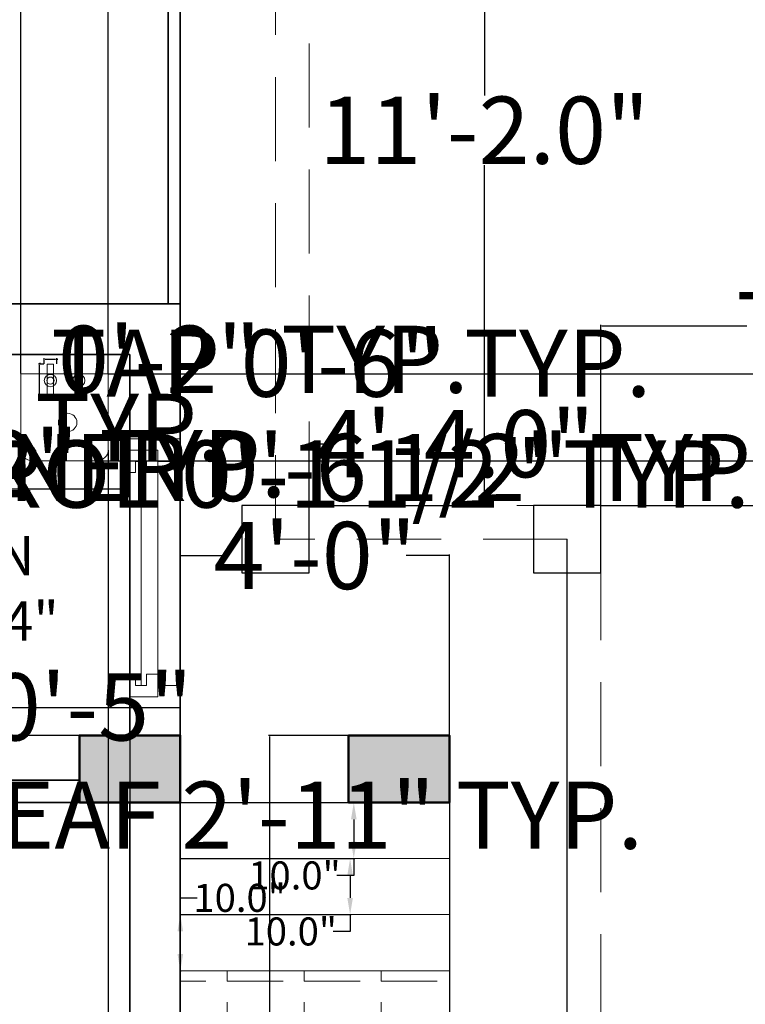
# Model space of a CAD drawing. Units: inches. Extents: x 1063 to 2718, y 423 to 1923.
# Tile 5 of 7: x 1379 to 1509, y 862 to 1038. Entities that reach past the tile are written whole.
import ezdxf

# ---------------------------------------------------------------- set-up
doc = ezdxf.new("R2010")
doc.units = ezdxf.units.IN
doc.header["$LTSCALE"] = 6
doc.header["$MEASUREMENT"] = 0
doc.linetypes.add('HIDDEN', pattern=[0.375, 0.25, -0.125])
for name, color, linetype, lineweight in [('A-ANNO-DIMS', 2, 'Continuous', 18), ('A-AREA-IDEN', 7, 'Continuous', 18), ('A-COLS', 7, 'Continuous', 50), ('A-COLS-PATT', 252, 'Continuous', 13), ('A-FLOR', 7, 'Continuous', 25), ('A-FLOR-CASE', 7, 'Continuous', 25), ('A-FLOR-FIXT', 4, 'Continuous', 18), ('A-FLOR-PATT', 9, 'Continuous', 13), ('A-FLOR-STRS', 7, 'Continuous', 18), ('A-GLAZ', 4, 'Continuous', 18), ('A-WALL', 7, 'Continuous', 35), ('C-PROP', 7, 'Continuous', 25), ('C-PROP-HIDN', 7, 'HIDDEN', 18)]:
    doc.layers.add(name, color=color, linetype=linetype, lineweight=lineweight)
doc.styles.get("Standard").update_dxf_attribs({"font": 'arial.ttf'})
doc.dimstyles.get("Standard").update_dxf_attribs({"dimtxt": 12, "dimasz": 0.18, "dimexe": 0.18, "dimexo": 0.0625, "dimgap": 0.09, "dimtad": 0, "dimtih": 1, "dimtoh": 1, "dimdec": 1, "dimzin": 0, "dimdsep": 46, "dimlunit": 3, "dimtxsty": 'Standard', "dimcen": 0.09, "dimadec": 0, "dimazin": 0, "dimtfac": 1, "dimtdec": 1, "dimtofl": 0, "dimtmove": 0, "dimatfit": 3, "dimfxl": 1, "dimtolj": 1, "dimtzin": 0, "dimarcsym": 0})

# ---------------------------------------------------------------- blocks, each defined once
blk = doc.blocks.new('*D3')
at = {"layer": 'A-ANNO-DIMS', "color": 0, "lineweight": -2, "ltscale": 6, "transparency": 16777216}
for p, q in [((1482.99, 951.12), (1516.18, 951.12)), ((1516, 950.94), (1516, 765.34)), ((1516, 567.3), (1516, 752.9)), ((1482.99, 567.12), (1516.18, 567.12))]:
    blk.add_line(p, q, dxfattribs=at)
at = {"layer": 'A-ANNO-DIMS', "color": 0, "ltscale": 6, "transparency": 16777216}
for points in [[(1515.97, 950.94), (1516.03, 950.94), (1516, 951.12)], [(1515.97, 567.3), (1516.03, 567.3), (1516, 567.12)]]:
    blk.add_solid(points, dxfattribs=at)
at = {"layer": 'Defpoints', "color": 0, "ltscale": 6, "transparency": 16777216}
for p in [(1482.93, 951.12), (1516, 951.12), (1482.93, 567.12)]:
    blk.add_point(p, dxfattribs=at)
at = {"layer": 'A-ANNO-DIMS', "color": 0, "ltscale": 6, "transparency": 16777216, "insert": (1516, 759.12), "char_height": 12, "attachment_point": 5}
blk.add_mtext("\\A1;32'", dxfattribs=at)
blk = doc.blocks.new('*D4')
at = {"layer": 'A-ANNO-DIMS', "color": 0, "lineweight": -2, "ltscale": 6, "transparency": 16777216}
for p, q in [((1430.93, 951.18), (1430.93, 962.35)), ((1431.11, 962.17), (1433.65, 962.17)), ((1482.75, 962.17), (1480.2, 962.17)), ((1482.93, 951.18), (1482.93, 962.35))]:
    blk.add_line(p, q, dxfattribs=at)
at = {"layer": 'A-ANNO-DIMS', "color": 0, "ltscale": 6, "transparency": 16777216}
for points in [[(1431.11, 962.2), (1431.11, 962.14), (1430.93, 962.17)], [(1482.75, 962.2), (1482.75, 962.14), (1482.93, 962.17)]]:
    blk.add_solid(points, dxfattribs=at)
at = {"layer": 'Defpoints', "color": 0, "ltscale": 6, "transparency": 16777216}
for p in [(1430.93, 962.17), (1430.93, 951.12), (1482.93, 951.12)]:
    blk.add_point(p, dxfattribs=at)
at = {"layer": 'A-ANNO-DIMS', "color": 0, "ltscale": 6, "transparency": 16777216, "insert": (1456.93, 962.17), "char_height": 12, "attachment_point": 5}
blk.add_mtext('\\A1;4\'-4.0"', dxfattribs=at)
blk = doc.blocks.new('*D5')
at = {"layer": 'A-ANNO-DIMS', "color": 0, "lineweight": -2, "ltscale": 6, "transparency": 16777216}
for p, q in [((1430.99, 1085.12), (1462.35, 1085.12)), ((1462.17, 1084.94), (1462.17, 1024.34)), ((1462.17, 951.3), (1462.17, 1011.9)), ((1430.99, 951.12), (1462.35, 951.12))]:
    blk.add_line(p, q, dxfattribs=at)
at = {"layer": 'A-ANNO-DIMS', "color": 0, "ltscale": 6, "transparency": 16777216}
for points in [[(1462.14, 1084.94), (1462.2, 1084.94), (1462.17, 1085.12)], [(1462.14, 951.3), (1462.2, 951.3), (1462.17, 951.12)]]:
    blk.add_solid(points, dxfattribs=at)
at = {"layer": 'Defpoints', "color": 0, "ltscale": 6, "transparency": 16777216}
for p in [(1430.93, 1085.12), (1462.17, 1085.12), (1430.93, 951.12)]:
    blk.add_point(p, dxfattribs=at)
at = {"layer": 'A-ANNO-DIMS', "color": 0, "ltscale": 6, "transparency": 16777216, "insert": (1462.17, 1018.12), "char_height": 12, "attachment_point": 5}
blk.add_mtext('\\A1;11\'-2.0"', dxfattribs=at)
blk = doc.blocks.new('*D8')
at = {"layer": 'A-ANNO-DIMS', "color": 0, "lineweight": -2, "ltscale": 6, "transparency": 16777216}
for p, q in [((1407.99, 898.12), (1439.05, 898.12)), ((1438.87, 895.12), (1438.87, 891.12)), ((1407.99, 888.12), (1439.05, 888.12)), ((1438.87, 888.12), (1438.87, 885.12)), ((1438.87, 885.12), (1435.87, 885.12))]:
    blk.add_line(p, q, dxfattribs=at)
at = {"layer": 'A-ANNO-DIMS', "color": 0, "ltscale": 6, "transparency": 16777216}
for points in [[(1438.37, 895.12), (1439.37, 895.12), (1438.87, 898.12)], [(1438.37, 891.12), (1439.37, 891.12), (1438.87, 888.12)]]:
    blk.add_solid(points, dxfattribs=at)
at = {"layer": 'Defpoints', "color": 0, "ltscale": 6, "transparency": 16777216}
for p in [(1407.93, 898.12), (1407.93, 888.12), (1438.87, 888.12)]:
    blk.add_point(p, dxfattribs=at)
at = {"layer": 'A-ANNO-DIMS', "color": 0, "ltscale": 6, "transparency": 16777216, "insert": (1428.29, 885.12), "char_height": 5, "attachment_point": 5}
blk.add_mtext('\\A1;10.0"', dxfattribs=at)
blk = doc.blocks.new('*D9')
at = {"layer": 'A-ANNO-DIMS', "color": 0, "lineweight": -2, "ltscale": 6, "transparency": 16777216}
for p, q in [((1407.99, 888.12), (1438.39, 888.12)), ((1438.21, 885.12), (1438.21, 881.12)), ((1407.99, 878.12), (1438.39, 878.12)), ((1438.21, 878.12), (1438.21, 875.12)), ((1438.21, 875.12), (1435.21, 875.12))]:
    blk.add_line(p, q, dxfattribs=at)
at = {"layer": 'A-ANNO-DIMS', "color": 0, "ltscale": 6, "transparency": 16777216}
for points in [[(1437.71, 885.12), (1438.71, 885.12), (1438.21, 888.12)], [(1437.71, 881.12), (1438.71, 881.12), (1438.21, 878.12)]]:
    blk.add_solid(points, dxfattribs=at)
at = {"layer": 'Defpoints', "color": 0, "ltscale": 6, "transparency": 16777216}
for p in [(1407.93, 888.12), (1407.93, 878.12), (1438.21, 878.12)]:
    blk.add_point(p, dxfattribs=at)
at = {"layer": 'A-ANNO-DIMS', "color": 0, "ltscale": 6, "transparency": 16777216, "insert": (1427.63, 875.12), "char_height": 5, "attachment_point": 5}
blk.add_mtext('\\A1;10.0"', dxfattribs=at)
blk = doc.blocks.new('*D10')
at = {"layer": 'A-ANNO-DIMS', "color": 0, "lineweight": -2, "ltscale": 6, "transparency": 16777216}
for p, q in [((1407.93, 878.12), (1407.93, 881.12)), ((1407.93, 881.12), (1410.93, 881.12)), ((1407.99, 878.12), (1408.11, 878.12)), ((1407.93, 871.12), (1407.93, 875.12)), ((1407.99, 868.12), (1408.11, 868.12))]:
    blk.add_line(p, q, dxfattribs=at)
at = {"layer": 'A-ANNO-DIMS', "color": 0, "ltscale": 6, "transparency": 16777216}
for points in [[(1407.43, 875.12), (1408.43, 875.12), (1407.93, 878.12)], [(1407.43, 871.12), (1408.43, 871.12), (1407.93, 868.12)]]:
    blk.add_solid(points, dxfattribs=at)
at = {"layer": 'Defpoints', "color": 0, "ltscale": 6, "transparency": 16777216}
for p in [(1407.93, 878.12), (1407.93, 878.12), (1407.93, 868.12)]:
    blk.add_point(p, dxfattribs=at)
at = {"layer": 'A-ANNO-DIMS', "color": 0, "ltscale": 6, "transparency": 16777216, "insert": (1418.51, 881.12), "char_height": 5, "attachment_point": 5}
blk.add_mtext('\\A1;10.0"', dxfattribs=at)
blk = doc.blocks.new('WIN-48-SLIDING')
at = {"ltscale": 6}
for p, q in [((0, 9), (4, 9)), ((4, 9), (4, 5)), ((48, 9), (44, 9)), ((44, 9), (44, 5)), ((4, 5), (2, 5)), ((2, 5), (2, 0)), ((4, 5), (44, 5)), ((4, 5), (6, 5)), ((6, 5), (6, 3)), ((44, 5), (42, 5)), ((42, 5), (42, 3)), ((44, 5), (46, 5)), ((46, 5), (46, 0)), ((6, 3), (4, 3)), ((4, 3), (4, 1)), ((4, 2), (44, 2)), ((42, 3), (44, 3)), ((44, 3), (44, 1)), ((4, 1), (6, 1)), ((6, 1), (6, 0)), ((44, 1), (42, 1)), ((42, 1), (42, 0)), ((48, 0), (0, 0)), ((2, 0), (46, 0))]:
    blk.add_line(p, q, dxfattribs=at)
blk.add_lwpolyline([(48, 0), (48, 9), (0, 9), (0, 0)], dxfattribs=at)
blk = doc.blocks.new('COLUMN-18X12')
blk.add_lwpolyline([(0, 0), (18, 0), (18, 12), (0, 12)], close=True)
blk = doc.blocks.new('PIER-12X12')
blk.add_lwpolyline([(0, 0), (12, 0), (12, 12), (0, 12)], close=True)
blk = doc.blocks.new('SINK-TAP')
at = {"ltscale": 6}
blk.add_lwpolyline([(0.54, 5.85), (1.67, 5.85), (1.67, 0), (0.54, 0)], close=True, dxfattribs=at)
for radius in [1.1, 1.1, 0.637]:
    blk.add_circle((1.1, 2.92), radius, dxfattribs=at)
blk = doc.blocks.new('*D34')
at = {"layer": 'A-ANNO-DIMS', "color": 0, "lineweight": -2, "ltscale": 6, "transparency": 16777216}
for p, q in [((1323.62, 956.91), (1323.62, 956.58)), ((1323.8, 956.76), (1324.88, 956.76)), ((1325.06, 956.91), (1325.06, 956.58)), ((1325.06, 956.76), (1325.24, 956.76))]:
    blk.add_line(p, q, dxfattribs=at)
at = {"layer": 'A-ANNO-DIMS', "color": 0, "ltscale": 6, "transparency": 16777216}
for points in [[(1323.8, 956.79), (1323.8, 956.73), (1323.62, 956.76)], [(1324.88, 956.79), (1324.88, 956.73), (1325.06, 956.76)]]:
    blk.add_solid(points, dxfattribs=at)
at = {"layer": 'Defpoints', "color": 0, "ltscale": 6, "transparency": 16777216}
for p in [(1323.62, 956.97), (1325.06, 956.97), (1325.06, 956.76)]:
    blk.add_point(p, dxfattribs=at)
at = {"layer": 'A-ANNO-DIMS', "color": 0, "ltscale": 6, "transparency": 16777216, "insert": (1419.12, 956.76), "char_height": 12, "attachment_point": 5}
blk.add_mtext('\\A1;CONTROL 0\'-1 1/2" TYP.', dxfattribs=at)
blk = doc.blocks.new('*D35')
at = {"layer": 'A-ANNO-DIMS', "color": 0, "lineweight": -2, "ltscale": 6, "transparency": 16777216}
for p, q in [((1325.12, 958.41), (1325.45, 958.41)), ((1325.27, 958.41), (1325.27, 958.59)), ((1325.27, 958.59), (1325.45, 958.59)), ((1325.27, 957.15), (1325.27, 958.23)), ((1325.12, 956.97), (1325.45, 956.97))]:
    blk.add_line(p, q, dxfattribs=at)
at = {"layer": 'A-ANNO-DIMS', "color": 0, "ltscale": 6, "transparency": 16777216}
for points in [[(1325.24, 958.23), (1325.3, 958.23), (1325.27, 958.41)], [(1325.24, 957.15), (1325.3, 957.15), (1325.27, 956.97)]]:
    blk.add_solid(points, dxfattribs=at)
at = {"layer": 'Defpoints', "color": 0, "ltscale": 6, "transparency": 16777216}
for p in [(1325.06, 958.41), (1325.27, 958.41), (1325.06, 956.97)]:
    blk.add_point(p, dxfattribs=at)
at = {"layer": 'A-ANNO-DIMS', "color": 0, "ltscale": 6, "transparency": 16777216, "insert": (1376.1, 958.59), "char_height": 12, "attachment_point": 5}
blk.add_mtext('\\A1;0\'-1 1/2" TYP.', dxfattribs=at)
blk = doc.blocks.new('*D36')
at = {"layer": 'A-ANNO-DIMS', "color": 0, "lineweight": -2, "ltscale": 6, "transparency": 16777216}
for p, q in [((1334.27, 958.87), (1334.27, 957.74)), ((1334.45, 957.92), (1340.83, 957.92)), ((1341.01, 958.87), (1341.01, 957.74)), ((1341.01, 957.92), (1341.19, 957.92))]:
    blk.add_line(p, q, dxfattribs=at)
at = {"layer": 'A-ANNO-DIMS', "color": 0, "ltscale": 6, "transparency": 16777216}
for points in [[(1334.45, 957.95), (1334.45, 957.89), (1334.27, 957.92)], [(1340.83, 957.95), (1340.83, 957.89), (1341.01, 957.92)]]:
    blk.add_solid(points, dxfattribs=at)
at = {"layer": 'Defpoints', "color": 0, "ltscale": 6, "transparency": 16777216}
for p in [(1334.27, 958.93), (1341.01, 958.93), (1341.01, 957.92)]:
    blk.add_point(p, dxfattribs=at)
at = {"layer": 'A-ANNO-DIMS', "color": 0, "ltscale": 6, "transparency": 16777216, "insert": (1429.29, 957.92), "char_height": 12, "attachment_point": 5}
blk.add_mtext('\\A1;BURNER 0\'-6 1/2" TYP.', dxfattribs=at)
blk = doc.blocks.new('*D37')
at = {"layer": 'A-ANNO-DIMS', "color": 0, "lineweight": -2, "ltscale": 6, "transparency": 16777216}
for p, q in [((1341.07, 964.9), (1342.2, 964.9)), ((1342.02, 964.9), (1342.02, 965.08)), ((1342.02, 965.08), (1342.2, 965.08)), ((1342.02, 959.11), (1342.02, 964.72)), ((1341.07, 958.93), (1342.2, 958.93))]:
    blk.add_line(p, q, dxfattribs=at)
at = {"layer": 'A-ANNO-DIMS', "color": 0, "ltscale": 6, "transparency": 16777216}
for points in [[(1341.99, 964.72), (1342.05, 964.72), (1342.02, 964.9)], [(1341.99, 959.11), (1342.05, 959.11), (1342.02, 958.93)]]:
    blk.add_solid(points, dxfattribs=at)
at = {"layer": 'Defpoints', "color": 0, "ltscale": 6, "transparency": 16777216}
for p in [(1341.01, 964.9), (1342.02, 964.9), (1341.01, 958.93)]:
    blk.add_point(p, dxfattribs=at)
at = {"layer": 'A-ANNO-DIMS', "color": 0, "ltscale": 6, "transparency": 16777216, "insert": (1378.86, 965.08), "char_height": 12, "attachment_point": 5}
blk.add_mtext('\\A1;0\'-6" TYP.', dxfattribs=at)
blk = doc.blocks.new('*D38')
at = {"layer": 'A-ANNO-DIMS', "color": 0, "lineweight": -2, "ltscale": 6, "transparency": 16777216}
for p, q in [((1383.61, 976.37), (1382.62, 976.37)), ((1382.8, 976.37), (1382.8, 976.55)), ((1382.8, 976.55), (1382.98, 976.55)), ((1382.8, 970.7), (1382.8, 976.19)), ((1383.61, 970.52), (1382.62, 970.52))]:
    blk.add_line(p, q, dxfattribs=at)
at = {"layer": 'A-ANNO-DIMS', "color": 0, "ltscale": 6, "transparency": 16777216}
for points in [[(1382.77, 976.19), (1382.83, 976.19), (1382.8, 976.37)], [(1382.77, 970.7), (1382.83, 970.7), (1382.8, 970.52)]]:
    blk.add_solid(points, dxfattribs=at)
at = {"layer": 'Defpoints', "color": 0, "ltscale": 6, "transparency": 16777216}
for p in [(1382.8, 976.37), (1383.67, 976.37), (1383.67, 970.52)]:
    blk.add_point(p, dxfattribs=at)
at = {"layer": 'A-ANNO-DIMS', "color": 0, "ltscale": 6, "transparency": 16777216, "insert": (1438.42, 976.55), "char_height": 12, "attachment_point": 5}
blk.add_mtext('\\A1;TAP 0\'-6" TYP.', dxfattribs=at)
blk = doc.blocks.new('*D39')
at = {"layer": 'A-ANNO-DIMS', "color": 0, "lineweight": -2, "ltscale": 6, "transparency": 16777216}
for p, q in [((1383.67, 976.43), (1383.67, 977.42)), ((1383.85, 977.24), (1385.7, 977.24)), ((1385.88, 976.43), (1385.88, 977.42)), ((1385.88, 977.24), (1386.06, 977.24))]:
    blk.add_line(p, q, dxfattribs=at)
at = {"layer": 'A-ANNO-DIMS', "color": 0, "ltscale": 6, "transparency": 16777216}
for points in [[(1383.85, 977.27), (1383.85, 977.21), (1383.67, 977.24)], [(1385.7, 977.27), (1385.7, 977.21), (1385.88, 977.24)]]:
    blk.add_solid(points, dxfattribs=at)
at = {"layer": 'Defpoints', "color": 0, "ltscale": 6, "transparency": 16777216}
for p in [(1385.88, 977.24), (1383.67, 976.37), (1385.88, 976.37)]:
    blk.add_point(p, dxfattribs=at)
at = {"layer": 'A-ANNO-DIMS', "color": 0, "ltscale": 6, "transparency": 16777216, "insert": (1422.73, 977.24), "char_height": 12, "attachment_point": 5}
blk.add_mtext('\\A1;0\'-2" TYP.', dxfattribs=at)
blk = doc.blocks.new('*D42')
at = {"layer": 'A-ANNO-DIMS', "color": 0, "lineweight": -2, "ltscale": 6, "transparency": 16777216}
for p, q in [((1265.93, 901.06), (1265.93, 895.69)), ((1300.93, 901.06), (1300.93, 895.69)), ((1266.11, 895.87), (1300.75, 895.87)), ((1300.93, 895.87), (1301.11, 895.87))]:
    blk.add_line(p, q, dxfattribs=at)
at = {"layer": 'A-ANNO-DIMS', "color": 0, "ltscale": 6, "transparency": 16777216}
for points in [[(1266.11, 895.9), (1266.11, 895.84), (1265.93, 895.87)], [(1300.75, 895.9), (1300.75, 895.84), (1300.93, 895.87)]]:
    blk.add_solid(points, dxfattribs=at)
at = {"layer": 'Defpoints', "color": 0, "ltscale": 6, "transparency": 16777216}
for p in [(1265.93, 901.12), (1300.93, 901.12), (1300.93, 895.87)]:
    blk.add_point(p, dxfattribs=at)
at = {"layer": 'A-ANNO-DIMS', "color": 0, "ltscale": 6, "transparency": 16777216, "insert": (1398.77, 895.87), "char_height": 12, "attachment_point": 5}
blk.add_mtext('\\A1;SINGLE LEAF 2\'-11" TYP.', dxfattribs=at)
blk = doc.blocks.new('*D48')
at = {"layer": 'A-ANNO-DIMS', "color": 0, "lineweight": -2, "ltscale": 6, "transparency": 16777216}
for p, q in [((1482.93, 951.18), (1482.93, 983.4)), ((1483.11, 983.22), (1508.94, 983.22)), ((1566.75, 983.22), (1540.92, 983.22)), ((1566.93, 951.18), (1566.93, 983.4))]:
    blk.add_line(p, q, dxfattribs=at)
at = {"layer": 'A-ANNO-DIMS', "color": 0, "ltscale": 6, "transparency": 16777216}
for points in [[(1483.11, 983.25), (1483.11, 983.19), (1482.93, 983.22)], [(1566.75, 983.25), (1566.75, 983.19), (1566.93, 983.22)]]:
    blk.add_solid(points, dxfattribs=at)
at = {"layer": 'Defpoints', "color": 0, "ltscale": 6, "transparency": 16777216}
for p in [(1566.93, 983.22), (1482.93, 951.12), (1566.93, 951.12)]:
    blk.add_point(p, dxfattribs=at)
at = {"layer": 'A-ANNO-DIMS', "color": 0, "ltscale": 6, "transparency": 16777216, "insert": (1524.93, 983.22), "char_height": 12, "attachment_point": 5}
blk.add_mtext('\\A1;7\'-0"', dxfattribs=at)
blk = doc.blocks.new('*D51')
at = {"layer": 'A-ANNO-DIMS', "color": 0, "lineweight": -2, "ltscale": 6, "transparency": 16777216}
for p, q in [((1407.93, 910.18), (1407.93, 942.4)), ((1408.11, 942.22), (1415.64, 942.22)), ((1455.75, 942.22), (1448.21, 942.22)), ((1455.93, 910.18), (1455.93, 942.4))]:
    blk.add_line(p, q, dxfattribs=at)
at = {"layer": 'A-ANNO-DIMS', "color": 0, "ltscale": 6, "transparency": 16777216}
for points in [[(1408.11, 942.25), (1408.11, 942.19), (1407.93, 942.22)], [(1455.75, 942.25), (1455.75, 942.19), (1455.93, 942.22)]]:
    blk.add_solid(points, dxfattribs=at)
at = {"layer": 'Defpoints', "color": 0, "ltscale": 6, "transparency": 16777216}
for p in [(1455.93, 942.22), (1407.93, 910.12), (1455.93, 910.12)]:
    blk.add_point(p, dxfattribs=at)
at = {"layer": 'A-ANNO-DIMS', "color": 0, "ltscale": 6, "transparency": 16777216, "insert": (1431.93, 942.22), "char_height": 12, "attachment_point": 5}
blk.add_mtext('\\A1;4\'-0"', dxfattribs=at)
blk = doc.blocks.new('*D52')
at = {"layer": 'A-ANNO-DIMS', "color": 0, "lineweight": -2, "ltscale": 6, "transparency": 16777216}
for p, q in [((1455.86, 910.12), (1423.65, 910.12)), ((1423.83, 909.94), (1423.83, 756.84)), ((1423.83, 591.3), (1423.83, 744.4)), ((1455.86, 591.12), (1423.65, 591.12))]:
    blk.add_line(p, q, dxfattribs=at)
at = {"layer": 'A-ANNO-DIMS', "color": 0, "ltscale": 6, "transparency": 16777216}
for points in [[(1423.8, 909.94), (1423.86, 909.94), (1423.83, 910.12)], [(1423.8, 591.3), (1423.86, 591.3), (1423.83, 591.12)]]:
    blk.add_solid(points, dxfattribs=at)
at = {"layer": 'Defpoints', "color": 0, "ltscale": 6, "transparency": 16777216}
for p in [(1423.83, 910.12), (1455.93, 910.12), (1455.93, 591.12)]:
    blk.add_point(p, dxfattribs=at)
at = {"layer": 'A-ANNO-DIMS', "color": 0, "ltscale": 6, "transparency": 16777216, "insert": (1423.83, 750.62), "char_height": 12, "attachment_point": 5}
blk.add_mtext('\\A1;26\'-7"', dxfattribs=at)
blk = doc.blocks.new('*D60')
at = {"layer": 'A-ANNO-DIMS', "color": 0, "lineweight": -2, "ltscale": 6, "transparency": 16777216}
for p, q in [((1321.21, 974.62), (1321.21, 1117.4)), ((1321.39, 1117.22), (1342.7, 1117.22)), ((1342.88, 974.62), (1342.88, 1117.4)), ((1342.88, 1117.22), (1343.06, 1117.22))]:
    blk.add_line(p, q, dxfattribs=at)
at = {"layer": 'A-ANNO-DIMS', "color": 0, "ltscale": 6, "transparency": 16777216}
for points in [[(1321.39, 1117.25), (1321.39, 1117.19), (1321.21, 1117.22)], [(1342.7, 1117.25), (1342.7, 1117.19), (1342.88, 1117.22)]]:
    blk.add_solid(points, dxfattribs=at)
at = {"layer": 'Defpoints', "color": 0, "ltscale": 6, "transparency": 16777216}
for p in [(1342.88, 1117.22), (1321.21, 974.55), (1342.88, 974.55)]:
    blk.add_point(p, dxfattribs=at)
at = {"layer": 'A-ANNO-DIMS', "color": 0, "ltscale": 6, "transparency": 16777216, "insert": (1372.52, 1117.22), "char_height": 12, "attachment_point": 5}
blk.add_mtext('\\A1;1\'-9 1/2"', dxfattribs=at)
blk = doc.blocks.new('*D62')
at = {"layer": 'A-ANNO-DIMS', "color": 0, "lineweight": -2, "ltscale": 6, "transparency": 16777216}
for p, q in [((1379.5, 974.73), (1379.5, 1117.4)), ((1379.68, 1117.22), (1394.9, 1117.22)), ((1395.08, 974.73), (1395.08, 1117.4)), ((1395.08, 1117.22), (1395.26, 1117.22))]:
    blk.add_line(p, q, dxfattribs=at)
at = {"layer": 'A-ANNO-DIMS', "color": 0, "ltscale": 6, "transparency": 16777216}
for points in [[(1379.68, 1117.25), (1379.68, 1117.19), (1379.5, 1117.22)], [(1394.9, 1117.25), (1394.9, 1117.19), (1395.08, 1117.22)]]:
    blk.add_solid(points, dxfattribs=at)
at = {"layer": 'Defpoints', "color": 0, "ltscale": 6, "transparency": 16777216}
for p in [(1395.08, 1117.22), (1379.5, 974.67), (1395.08, 974.67)]:
    blk.add_point(p, dxfattribs=at)
at = {"layer": 'A-ANNO-DIMS', "color": 0, "ltscale": 6, "transparency": 16777216, "insert": (1424.71, 1117.22), "char_height": 12, "attachment_point": 5}
blk.add_mtext('\\A1;1\'-3 1/2"', dxfattribs=at)
blk = doc.blocks.new('*D63')
at = {"layer": 'A-ANNO-DIMS', "color": 0, "lineweight": -2, "ltscale": 6, "transparency": 16777216}
for p, q in [((1395.14, 974.67), (1599.21, 974.67)), ((1599.03, 974.49), (1599.03, 973.19)), ((1599.03, 959.29), (1599.03, 960.59)), ((1393.14, 959.11), (1599.21, 959.11))]:
    blk.add_line(p, q, dxfattribs=at)
at = {"layer": 'A-ANNO-DIMS', "color": 0, "ltscale": 6, "transparency": 16777216}
for points in [[(1599, 974.49), (1599.06, 974.49), (1599.03, 974.67)], [(1599, 959.29), (1599.06, 959.29), (1599.03, 959.11)]]:
    blk.add_solid(points, dxfattribs=at)
at = {"layer": 'Defpoints', "color": 0, "ltscale": 6, "transparency": 16777216}
for p in [(1395.08, 974.67), (1393.08, 959.11), (1599.03, 959.11)]:
    blk.add_point(p, dxfattribs=at)
at = {"layer": 'A-ANNO-DIMS', "color": 0, "ltscale": 6, "transparency": 16777216, "insert": (1599.03, 966.89), "char_height": 12, "attachment_point": 5}
blk.add_mtext('\\A1;1\'-3 1/2"', dxfattribs=at)
blk = doc.blocks.new('*D64')
at = {"layer": 'A-ANNO-DIMS', "color": 0, "lineweight": -2, "ltscale": 6, "transparency": 16777216}
for p, q in [((1310.93, 978.18), (1310.93, 1117.4)), ((1311.11, 1117.22), (1321.03, 1117.22)), ((1321.21, 974.62), (1321.21, 1117.4)), ((1321.21, 1117.22), (1321.39, 1117.22))]:
    blk.add_line(p, q, dxfattribs=at)
at = {"layer": 'A-ANNO-DIMS', "color": 0, "ltscale": 6, "transparency": 16777216}
for points in [[(1311.11, 1117.25), (1311.11, 1117.19), (1310.93, 1117.22)], [(1321.03, 1117.25), (1321.03, 1117.19), (1321.21, 1117.22)]]:
    blk.add_solid(points, dxfattribs=at)
at = {"layer": 'Defpoints', "color": 0, "ltscale": 6, "transparency": 16777216}
for p in [(1321.21, 1117.22), (1310.93, 978.12), (1321.21, 974.55)]:
    blk.add_point(p, dxfattribs=at)
at = {"layer": 'A-ANNO-DIMS', "color": 0, "ltscale": 6, "transparency": 16777216, "insert": (1356.07, 1117.22), "char_height": 12, "attachment_point": 5}
blk.add_mtext('\\A1;0\'-10 1/2"', dxfattribs=at)
blk = doc.blocks.new('*D65')
at = {"layer": 'A-ANNO-DIMS', "color": 0, "lineweight": -2, "ltscale": 6, "transparency": 16777216}
for p, q in [((1395.08, 961.04), (1395.08, 431.18)), ((1398.93, 954.06), (1398.93, 431.18)), ((1395.26, 431.36), (1398.75, 431.36)), ((1398.93, 431.36), (1399.11, 431.36))]:
    blk.add_line(p, q, dxfattribs=at)
at = {"layer": 'A-ANNO-DIMS', "color": 0, "ltscale": 6, "transparency": 16777216}
for points in [[(1395.26, 431.39), (1395.26, 431.33), (1395.08, 431.36)], [(1398.75, 431.39), (1398.75, 431.33), (1398.93, 431.36)]]:
    blk.add_solid(points, dxfattribs=at)
at = {"layer": 'Defpoints', "color": 0, "ltscale": 6, "transparency": 16777216}
for p in [(1395.08, 961.11), (1398.93, 954.12), (1398.93, 431.36)]:
    blk.add_point(p, dxfattribs=at)
at = {"layer": 'A-ANNO-DIMS', "color": 0, "ltscale": 6, "transparency": 16777216, "insert": (1415.15, 431.36), "char_height": 12, "attachment_point": 5}
blk.add_mtext('\\A1;0\'-4"', dxfattribs=at)
blk = doc.blocks.new('*D72')
at = {"layer": 'A-ANNO-DIMS', "color": 0, "lineweight": -2, "ltscale": 6, "transparency": 16777216}
for p, q in [((1407.86, 915.02), (1375.65, 915.02)), ((1375.83, 915.02), (1375.83, 915.2)), ((1375.83, 915.2), (1376.01, 915.2)), ((1375.83, 910.3), (1375.83, 914.84)), ((1407.86, 910.12), (1375.65, 910.12))]:
    blk.add_line(p, q, dxfattribs=at)
at = {"layer": 'A-ANNO-DIMS', "color": 0, "ltscale": 6, "transparency": 16777216}
for points in [[(1375.8, 914.84), (1375.86, 914.84), (1375.83, 915.02)], [(1375.8, 910.3), (1375.86, 910.3), (1375.83, 910.12)]]:
    blk.add_solid(points, dxfattribs=at)
at = {"layer": 'Defpoints', "color": 0, "ltscale": 6, "transparency": 16777216}
for p in [(1375.83, 915.02), (1407.93, 915.02), (1407.93, 910.12)]:
    blk.add_point(p, dxfattribs=at)
at = {"layer": 'A-ANNO-DIMS', "color": 0, "ltscale": 6, "transparency": 16777216, "insert": (1392.05, 915.2), "char_height": 12, "attachment_point": 5}
blk.add_mtext('\\A1;0\'-5"', dxfattribs=at)

msp = doc.modelspace()

# ---------------------------------------------------------------- hatches: boundary and pattern name
at = {"layer": 'A-COLS-PATT', "ltscale": 6}
h = msp.add_hatch(color=256, dxfattribs=at)
h.dxf.hatch_style = 1
h.paths.add_polyline_path([(1192.93, 603.12), (1174.93, 603.12), (1174.93, 591.12), (1192.93, 591.12)])
h.paths.add_polyline_path([(1407.93, 603.12), (1389.93, 603.12), (1389.93, 591.12), (1407.93, 591.12)])
h.paths.add_polyline_path([(1192.93, 756.12), (1174.93, 756.12), (1174.93, 744.12), (1192.93, 744.12)])
h.paths.add_polyline_path([(1407.93, 761.11), (1389.93, 761.11), (1389.93, 749.11), (1407.93, 749.11)])
h.paths.add_polyline_path([(1455.93, 761.11), (1437.93, 761.11), (1437.93, 749.11), (1455.93, 749.11)])
h.paths.add_polyline_path([(1455.93, 910.12), (1437.93, 910.12), (1437.93, 898.12), (1455.93, 898.12)])
h.paths.add_polyline_path([(1407.93, 910.12), (1389.93, 910.12), (1389.93, 898.12), (1407.93, 898.12)])
h.paths.add_polyline_path([(1192.93, 910.12), (1174.93, 910.12), (1174.93, 898.12), (1192.93, 898.12)])
h.paths.add_polyline_path([(1192.93, 1055.12), (1174.93, 1055.12), (1174.93, 1043.12), (1192.93, 1043.12)])
h.paths.add_polyline_path([(1407.93, 1055.12), (1389.93, 1055.12), (1389.93, 1043.12), (1407.93, 1043.12)])
at = {"layer": 'A-FLOR-PATT', "ltscale": 6}
h = msp.add_hatch(dxfattribs=at)
h.set_pattern_fill('ANGLE', color=256, scale=50)
h.set_pattern_definition([(0, (0, 0), (0, 13.75), [10, -3.75]), (90, (0, 0), (-13.75, 8e-16), [10, -3.75])])
h.paths.add_polyline_path([(1455.93, 749.11), (1437.93, 749.11), (1437.93, 761.11), (1455.93, 761.11), (1455.93, 868.12), (1407.93, 868.12), (1407.93, 595.12), (1455.93, 595.12)])
h.paths.add_polyline_path([(1377.93, 674.12), (1315.93, 674.12), (1315.93, 600.12), (1377.93, 600.12)])

# ---------------------------------------------------------------- linework, layer by layer
at = {"layer": 'A-FLOR'}
for p, q in [((1407.93, 898.12), (1455.93, 898.12)), ((1455.93, 898.12), (1455.93, 591.12))]:
    msp.add_line(p, q, dxfattribs=at)
at = {"layer": 'A-FLOR-CASE'}
msp.add_line((1310.93, 954.12), (1398.93, 954.12), dxfattribs=at)
at = {"layer": 'A-FLOR-FIXT', "ltscale": 6}
for p, q in [((1379.5, 974.67), (1395.08, 974.67)), ((1379.5, 974.67), (1379.5, 961.11)), ((1395.08, 974.67), (1395.08, 961.11)), ((1393.08, 959.11), (1381.5, 959.11))]:
    msp.add_line(p, q, dxfattribs=at)
msp.add_circle((1387.84, 965.96), 1.64, dxfattribs=at)
for centre, start, end in [((1381.5, 961.11), 180, 270), ((1393.08, 961.11), 270, 0)]:
    msp.add_arc(centre, 2, start, end, dxfattribs=at)
at = {"layer": 'A-FLOR-STRS'}
for p, q in [((1407.93, 888.12), (1455.93, 888.12)), ((1407.93, 878.12), (1455.93, 878.12)), ((1407.93, 868.12), (1455.93, 868.12))]:
    msp.add_line(p, q, dxfattribs=at)
at = {"layer": 'A-WALL', "ltscale": 6}
for p, q in [((1407.93, 1055.12), (1407.93, 591.12)), ((1389.93, 902.12), (1350.93, 902.12)), ((1350.46, 898.12), (1398.93, 898.12))]:
    msp.add_line(p, q, dxfattribs=at)
at = {"layer": 'A-WALL'}
for p, q in [((1405.75, 1043.12), (1405.75, 987.12)), ((1315.75, 987.12), (1407.93, 987.12)), ((1310.93, 978.12), (1398.93, 978.12)), ((1398.93, 978.12), (1398.93, 910.12)), ((1398.93, 898.12), (1398.93, 842.62))]:
    msp.add_line(p, q, dxfattribs=at)
at = {"layer": 'C-PROP'}
msp.add_line((1476.93, 567.12), (1476.93, 945.12), dxfattribs=at)
at = {"layer": 'C-PROP-HIDN', "ltscale": 10}
for p, q in [((1430.93, 951.12), (1430.93, 1085.12)), ((1424.93, 945.12), (1424.93, 1079.12)), ((1482.93, 951.12), (1430.93, 951.12)), ((1482.93, 567.12), (1482.93, 951.12)), ((1476.93, 945.12), (1424.93, 945.12))]:
    msp.add_line(p, q, dxfattribs=at)

# ---------------------------------------------------------------- block references
at = {"layer": 'A-COLS'}
for p in [(1389.93, 898.12), (1437.93, 898.12)]:
    msp.add_blockref('COLUMN-18X12', p, dxfattribs=at)
at = {"layer": 'A-FLOR-FIXT'}
msp.add_blockref('SINK-TAP', (1383.67, 970.52), dxfattribs=at)
at = {"layer": 'A-FLOR-FIXT', "extrusion": (0, 0, -1), "zscale": -1}
msp.add_blockref('SINK-TAP', (-1390.91, 970.52), dxfattribs=at)
at = {"layer": 'A-GLAZ', "rotation": 269.9999999999989}
msp.add_blockref('WIN-48-SLIDING', (1398.93, 963.02), dxfattribs=at)
at = {"layer": 'C-PROP'}
for p in [(1418.93, 939.12), (1470.93, 939.12)]:
    msp.add_blockref('PIER-12X12', p, dxfattribs=at)

# ---------------------------------------------------------------- texts
at = {"layer": 'A-AREA-IDEN', "ltscale": 6, "insert": (1341.66, 945.7), "char_height": 7, "attachment_point": 1}
msp.add_mtext_dynamic_manual_height_columns('KITCHEN\\P7\'4" x 6\'4"', width=175.2385, gutter_width=1, heights=[0], dxfattribs=at)

# ---------------------------------------------------------------- dimensions: what is measured, and where the dimension line sits
at = {"layer": 'A-ANNO-DIMS', "ltscale": 6}
for base, p1, p2, override, picture, middle in [((1321.21, 1117.22), (1310.93, 978.12), (1321.21, 974.55), {"dimdec": 1, "dimlfac": 1, "dimrnd": 0, "dimzin": 1, "dimdsep": 46, "dimlunit": 4, "dimfrac": 2}, '*D64', (1356.07, 1117.22)), ((1342.88, 1117.22), (1321.21, 974.55), (1342.88, 974.55), {"dimdec": 1, "dimlfac": 1, "dimrnd": 0, "dimzin": 1, "dimdsep": 46, "dimlunit": 4, "dimfrac": 2}, '*D60', (1372.52, 1117.22)), ((1395.08, 1117.22), (1379.5, 974.67), (1395.08, 974.67), {"dimdec": 1, "dimlfac": 1, "dimrnd": 0, "dimzin": 1, "dimdsep": 46, "dimlunit": 4, "dimfrac": 2}, '*D62', (1424.71, 1117.22)), ((1430.93, 962.17), (1482.93, 951.12), (1430.93, 951.12), {"dimclrd": 0, "dimclre": 0, "dimclrt": 0}, '*D4', (1456.93, 962.17)), ((1398.9256, 431.3553), (1395.0779, 961.1073), (1398.9256, 954.1189), {"dimdec": 1, "dimlfac": 1, "dimrnd": 0, "dimzin": 1, "dimdsep": 46, "dimlunit": 4, "dimfrac": 2}, '*D65', (1415.1451, 431.3553)), ((1455.93, 942.22), (1407.93, 910.12), (1455.93, 910.12), {"dimdec": 1, "dimlfac": 1, "dimrnd": 0, "dimzin": 1, "dimdsep": 46, "dimlunit": 4, "dimfrac": 2}, '*D51', (1431.93, 942.22))]:
    dim = msp.add_linear_dim(base=base, p1=p1, p2=p2, dimstyle='Standard', override=override, dxfattribs=at)
    dim.commit()
    dim.dimension.update_dxf_attribs({"geometry": picture, "text_midpoint": middle})
for base, p1, p2, angle, override, picture, middle in [((1462.17, 1085.12), (1430.93, 951.12), (1430.93, 1085.12), 90, {"dimclrd": 0, "dimclre": 0, "dimclrt": 0}, '*D5', (1462.17, 1018.12)), ((1566.93, 983.22), (1482.93, 951.12), (1566.93, 951.12), 0, {"dimdec": 1, "dimlfac": 1, "dimrnd": 0, "dimzin": 1, "dimdsep": 46, "dimlunit": 4, "dimfrac": 2}, '*D48', (1524.93, 983.22)), ((1599.03, 959.11), (1395.08, 974.67), (1393.08, 959.11), 90, {"dimdec": 1, "dimlfac": 1, "dimrnd": 0, "dimzin": 1, "dimdsep": 46, "dimlunit": 4, "dimfrac": 2}, '*D63', (1599.03, 966.89)), ((1516, 951.12), (1482.93, 567.12), (1482.93, 951.12), 90, {"dimclrd": 0, "dimclre": 0, "dimclrt": 0}, '*D3', (1516, 759.12)), ((1375.83, 915.02), (1407.93, 910.12), (1407.93, 915.02), 90, {"dimdec": 1, "dimlfac": 1, "dimrnd": 0, "dimzin": 1, "dimdsep": 46, "dimlunit": 4, "dimfrac": 2}, '*D72', (1392.05, 915.2)), ((1423.83, 910.12), (1455.93, 591.12), (1455.93, 910.12), 90, {"dimdec": 1, "dimlfac": 1, "dimrnd": 0, "dimzin": 1, "dimdsep": 46, "dimlunit": 4, "dimfrac": 2}, '*D52', (1423.83, 750.62)), ((1438.87, 888.12), (1407.93, 898.12), (1407.93, 888.12), 90, {"dimtxt": 5, "dimasz": 3, "dimclrd": 0, "dimclre": 0, "dimclrt": 0}, '*D8', (1428.29, 885.12)), ((1438.21, 878.12), (1407.93, 888.12), (1407.93, 878.12), 90, {"dimtxt": 5, "dimasz": 3, "dimclrd": 0, "dimclre": 0, "dimclrt": 0}, '*D9', (1427.63, 875.12)), ((1407.93, 878.12), (1407.93, 868.12), (1407.93, 878.12), 90, {"dimtxt": 5, "dimasz": 3, "dimclrd": 0, "dimclre": 0, "dimclrt": 0}, '*D10', (1418.51, 881.12))]:
    dim = msp.add_linear_dim(base=base, p1=p1, p2=p2, angle=angle, dimstyle='Standard', override=override, dxfattribs=at)
    dim.commit()
    dim.dimension.update_dxf_attribs({"geometry": picture, "text_midpoint": middle})
for base, p1, p2, text, picture, middle in [((1382.7976, 976.3667), (1383.6749, 970.5176), (1383.6749, 976.3667), 'TAP <> TYP.', '*D38', (1438.4223, 976.5467)), ((1325.27, 958.41), (1325.06, 956.97), (1325.06, 958.41), '<> TYP.', '*D35', (1376.1, 958.59)), ((1342.02, 964.9), (1341.01, 958.93), (1341.01, 964.9), '<> TYP.', '*D37', (1378.86, 965.08))]:
    dim = msp.add_linear_dim(base=base, p1=p1, p2=p2, angle=90, text=text, dimstyle='Standard', override={"dimdec": 1, "dimlfac": 1, "dimrnd": 0, "dimzin": 1, "dimdsep": 46, "dimlunit": 4, "dimfrac": 2}, dxfattribs=at)
    dim.commit()
    dim.dimension.update_dxf_attribs({"geometry": picture, "text_midpoint": middle})
for base, p1, p2, text, picture, middle in [((1325.06, 956.76), (1323.62, 956.97), (1325.06, 956.97), 'CONTROL <> TYP.', '*D34', (1419.12, 956.76)), ((1341.01, 957.92), (1334.27, 958.93), (1341.01, 958.93), 'BURNER <> TYP.', '*D36', (1429.29, 957.92)), ((1385.88, 977.24), (1383.67, 976.37), (1385.88, 976.37), '<> TYP.', '*D39', (1422.73, 977.24)), ((1300.93, 895.87), (1265.93, 901.12), (1300.93, 901.12), 'SINGLE LEAF <> TYP.', '*D42', (1398.77, 895.87))]:
    dim = msp.add_linear_dim(base=base, p1=p1, p2=p2, text=text, dimstyle='Standard', override={"dimdec": 1, "dimlfac": 1, "dimrnd": 0, "dimzin": 1, "dimdsep": 46, "dimlunit": 4, "dimfrac": 2}, dxfattribs=at)
    dim.commit()
    dim.dimension.update_dxf_attribs({"geometry": picture, "text_midpoint": middle})

doc.saveas('drawing.dxf')
